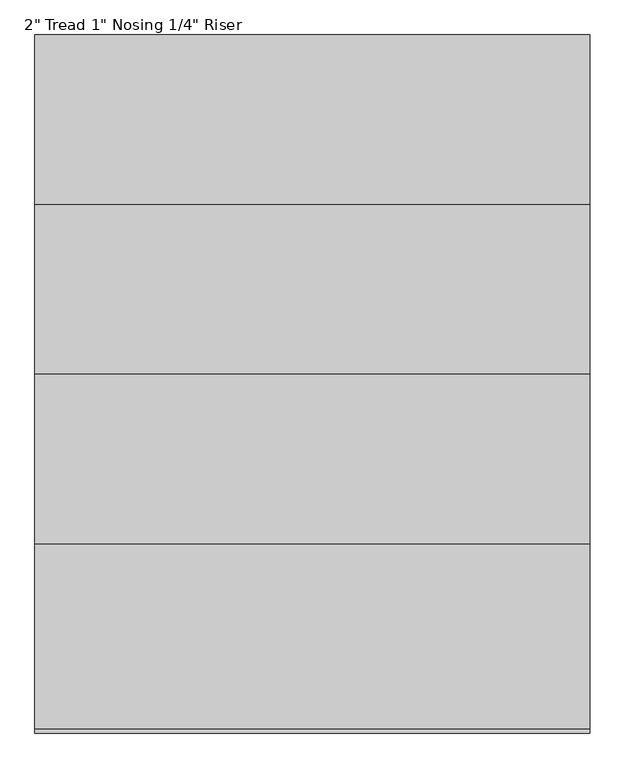
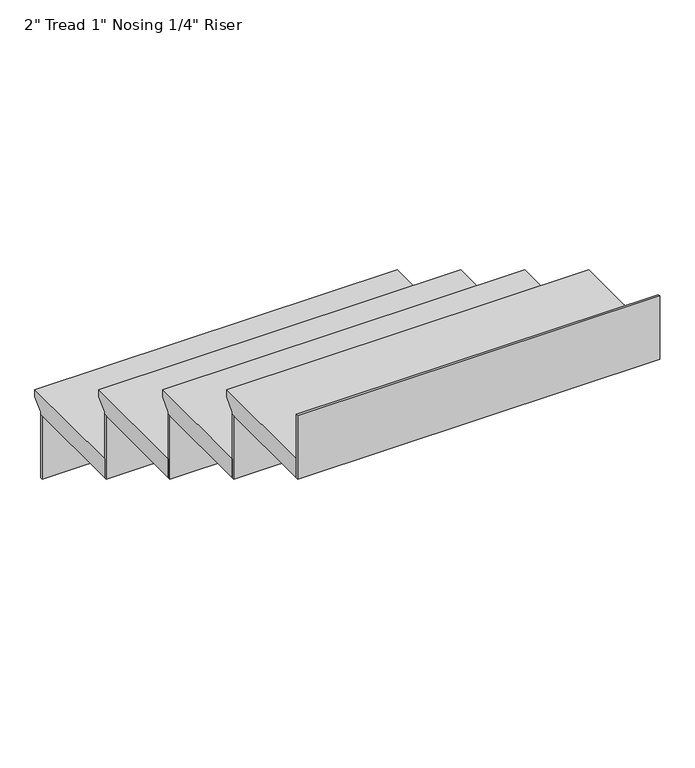
"""IFC4 building model written with IfcOpenShell, lengths in millimetres: stair flight geometry."""

from ifc_helpers import new_model, si_unit, frame, origin, place, context, project, spatial, polyline, outline, extrude, source, transform, mapped, element, save


def stair_flight_01bb6bd9(model_context):
    return source(origin(), model_context, "Body", "SweptSolid", [
        extrude(outline(polyline([(22889.9216096, 30653.2839133), (23194.7216096, 30653.2839133), (23194.7216096, 30634.2339133), (23169.3216096, 30608.8339133), (23169.3216096, 30602.4839133), (22889.9216096, 30602.4839133), (22889.9216096, 30653.2839133)])), frame((-2398.2415084, 0.0, 0.0), z_axis=(1.0, 0.0, 0.0), x_axis=(0.0, 1.0, 0.0)), (0.0, 0.0, 1.0), 914.4),
        extrude(outline(polyline([(-2398.2415084, 23162.9716096), (-2398.2415084, 23169.3216096), (-1483.8415084, 23169.3216096), (-1483.8415084, 23162.9716096), (-2398.2415084, 23162.9716096)])), frame((0.0, 0.0, 30433.1505799), z_axis=(0.0, 0.0, 1.0), x_axis=(1.0, 0.0, 0.0)), (0.0, 0.0, 1.0), 169.3333333),
        extrude(outline(polyline([(-2398.2415084, 22883.5716096), (-2398.2415084, 22889.9216096), (-1483.8415084, 22889.9216096), (-1483.8415084, 22883.5716096), (-2398.2415084, 22883.5716096)])), frame((0.0, 0.0, 30602.4839133), z_axis=(0.0, 0.0, 1.0), x_axis=(1.0, 0.0, 0.0)), (0.0, 0.0, 1.0), 169.3333333),
        extrude(outline(polyline([(22610.5216096, 30822.6172466), (22915.3216096, 30822.6172466), (22915.3216096, 30803.5672466), (22889.9216096, 30778.1672466), (22889.9216096, 30771.8172466), (22610.5216096, 30771.8172466), (22610.5216096, 30822.6172466)])), frame((-2398.2415084, 0.0, 0.0), z_axis=(1.0, 0.0, 0.0), x_axis=(0.0, 1.0, 0.0)), (0.0, 0.0, 1.0), 914.4),
        extrude(outline(polyline([(-2398.2415084, 22604.1716096), (-2398.2415084, 22610.5216096), (-1483.8415084, 22610.5216096), (-1483.8415084, 22604.1716096), (-2398.2415084, 22604.1716096)])), frame((0.0, 0.0, 30771.8172466), z_axis=(0.0, 0.0, 1.0), x_axis=(1.0, 0.0, 0.0)), (0.0, 0.0, 1.0), 169.3333333),
        extrude(outline(polyline([(22331.1216096, 30991.9505799), (22635.9216096, 30991.9505799), (22635.9216096, 30972.9005799), (22610.5216096, 30947.5005799), (22610.5216096, 30941.1505799), (22331.1216096, 30941.1505799), (22331.1216096, 30991.9505799)])), frame((-2398.2415084, 0.0, 0.0), z_axis=(1.0, 0.0, 0.0), x_axis=(0.0, 1.0, 0.0)), (0.0, 0.0, 1.0), 914.4),
        extrude(outline(polyline([(-2398.2415084, 22324.7716096), (-2398.2415084, 22331.1216096), (-1483.8415084, 22331.1216096), (-1483.8415084, 22324.7716096), (-2398.2415084, 22324.7716096)])), frame((0.0, 0.0, 30941.1505799), z_axis=(0.0, 0.0, 1.0), x_axis=(1.0, 0.0, 0.0)), (0.0, 0.0, 1.0), 169.3333333),
        extrude(outline(polyline([(-2398.2415084, 22045.3716096), (-2398.2415084, 22051.7216096), (-1483.8415084, 22051.7216096), (-1483.8415084, 22045.3716096), (-2398.2415084, 22045.3716096)])), frame((0.0, 0.0, 31110.4839133), z_axis=(0.0, 0.0, 1.0), x_axis=(1.0, 0.0, 0.0)), (0.0, 0.0, 1.0), 169.3333333),
        extrude(outline(polyline([(22051.7216096, 31161.2839133), (22356.5216096, 31161.2839133), (22356.5216096, 31142.2339133), (22331.1216096, 31116.8339133), (22331.1216096, 31110.4839133), (22051.7216096, 31110.4839133), (22051.7216096, 31161.2839133)])), frame((-2398.2415084, 0.0, 0.0), z_axis=(1.0, 0.0, 0.0), x_axis=(0.0, 1.0, 0.0)), (0.0, 0.0, 1.0), 914.4),
    ])


if __name__ == "__main__":
    model = new_model("IFC4")
    model_context = context("Model", 3, world=origin())
    ifc_project = project(units=[si_unit("LENGTHUNIT", "METRE", prefix="MILLI")], contexts=[model_context])
    site = spatial("IfcSite", under=ifc_project)
    building = spatial("IfcBuilding", under=site)
    placement = place(None, origin())
    stair_flight_shape = stair_flight_01bb6bd9(model_context)
    element("IfcStairFlight", 1, ObjectType="2\" Tread 1\" Nosing 1/4\" Riser", at=placement, inside=building, context=model_context, shape_type="MappedRepresentation", body=[
        mapped(stair_flight_shape, transform((0.0, 0.0, 0.0), x_axis=(1.0, 0.0, 0.0), y_axis=(0.0, 1.0, 0.0), z_axis=(0.0, 0.0, 1.0))),
    ])
    save(model, "model.ifc")
